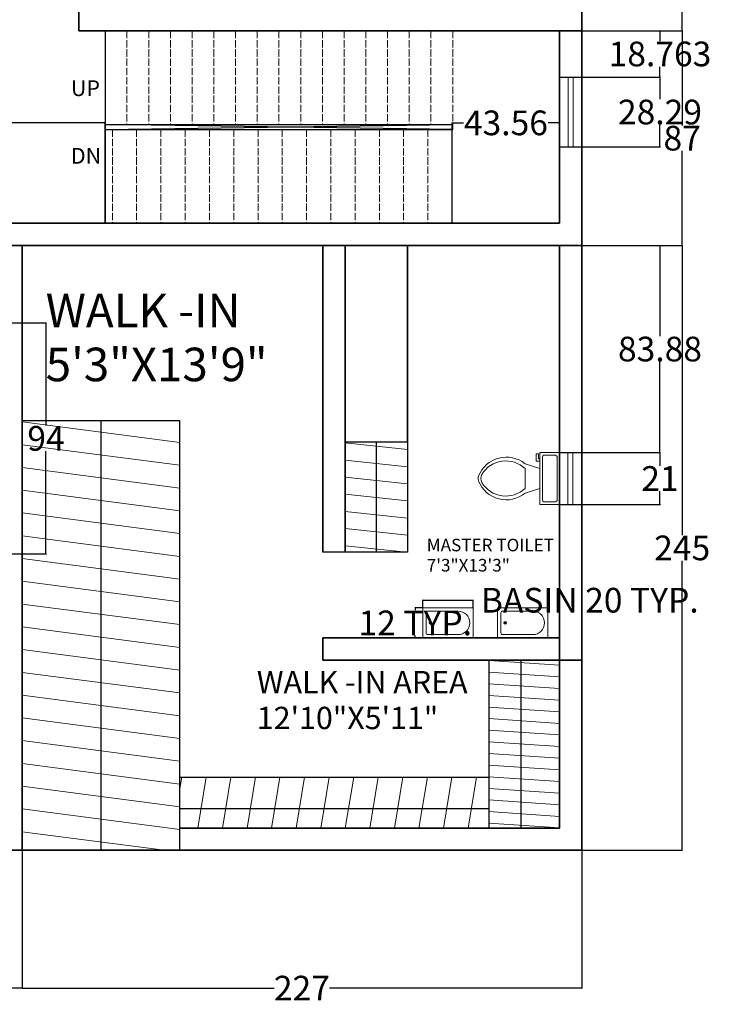
# Model space of a CAD drawing. Units: inches. Extents: x 135 to 880, y 60 to 879.
# Tile 3 of 5: x 557 to 838, y 60 to 459. Entities that reach past the tile are written whole.
import ezdxf

# ---------------------------------------------------------------- set-up
doc = ezdxf.new("R2010")
doc.units = ezdxf.units.IN
doc.header["$MEASUREMENT"] = 0
doc.linetypes.add('ACAD_ISO02W100', pattern=[15, 12, -3])
for name, color, linetype, lineweight in [('A-ANNO-DIMS', 2, 'Continuous', 18), ('A-ANNO-TEXT', 7, 'Continuous', 18), ('A-AREA-IDEN', 7, 'Continuous', 18), ('A-FLOR-CASE', 32, 'Continuous', 25), ('A-FLOR-CASE-PATT', 252, 'Continuous', 13), ('A-FLOR-FIXT', 9, 'Continuous', 20), ('A-FLOR-STRS', 7, 'Continuous', 25), ('A-FLOR-STRS-HIDN', 8, 'ACAD_ISO02W100', 18), ('A-GLAZ', 4, 'Continuous', 18), ('A-WALL', 7, 'Continuous', 35)]:
    doc.layers.add(name, color=color, linetype=linetype, lineweight=lineweight)
doc.styles.get("Standard").update_dxf_attribs({"font": 'arial.ttf'})
doc.dimstyles.get("Standard").update_dxf_attribs({"dimtxt": 10, "dimasz": 0.18, "dimexe": 0.18, "dimexo": 0.0625, "dimgap": 0.09, "dimtad": 0, "dimtih": 1, "dimtoh": 1, "dimdec": 0, "dimzin": 0, "dimdsep": 46, "dimlunit": 3, "dimtxsty": 'Standard', "dimcen": 0.09, "dimadec": 0, "dimazin": 0, "dimtfac": 1, "dimtdec": 0, "dimtofl": 0, "dimtmove": 0, "dimatfit": 3, "dimfxl": 1, "dimtolj": 1, "dimtzin": 0, "dimarcsym": 0})

# ---------------------------------------------------------------- blocks, each defined once
blk = doc.blocks.new('Toilet - top')
for p, q in [((9.5, -6), (9.5, -2)), ((-10, -8.5), (-8, -8.5)), ((-10, -9.5), (-10, -8.5)), ((-7, -9.5), (-10, -9.5)), ((-8, -8.5), (-8, -8)), ((-7, -8), (-7, -9.5)), ((-4, -8), (-6, -14)), ((4, -8), (6, -14)), ((4, -14), (-4, -14))]:
    blk.add_line(p, q)
blk.add_lwpolyline([(10.5, -8), (10.5, 0), (-10.5, 0), (-10.5, -8)], close=True)
for points in [[(-9.5, -2), (-9.5, -6)], [(8.5, -1), (-8.5, -1)], [(-8.5, -7), (8.5, -7)]]:
    blk.add_lwpolyline(points)
for centre, radius, start, end in [((-8.62, -1.88), 0.884, 81.8699, 188.1301), ((8.62, -1.88), 0.884, 351.8699, 98.1301), ((-8.62, -6.12), 0.884, 171.8699, 278.1301), ((8.62, -6.12), 0.884, 261.8699, 8.1301), ((3.52, -21.58), 12.17, 141.4691, 247.9714), ((4.2, -21.82), 11.33, 136.3677, 238.9468), ((-3.52, -21.58), 12.17, 292.0284, 38.5307), ((-4.2, -21.82), 11.33, 301.053, 43.6321), ((0, -27.88), 4, 245.7318, 294.2682), ((0, -29), 4, 254.8605, 285.1395)]:
    blk.add_arc(centre, radius, start, end)
blk = doc.blocks.new('Bath Tub - 26 x 60 in.')
for p, q in [((8, -18), (10, -18)), ((9, -17), (9, -19))]:
    blk.add_line(p, q)
blk.add_lwpolyline([(0, -36), (0, 0), (60, 0), (60, -36)], close=True)
for points in [[(4, -30), (4, -6)], [(6, -4), (42, -4)], [(42, -32), (6, -32)]]:
    blk.add_lwpolyline(points)
for radius in [1.5, 1]:
    blk.add_circle((9, -18), radius)
for centre, radius, start, end in [((5.75, -5.75), 1.77, 81.8699, 188.1301), ((42, -18), 14, 270, 90), ((5.75, -30.25), 1.77, 171.8699, 278.1301)]:
    blk.add_arc(centre, radius, start, end)
blk = doc.blocks.new('*D22')
at = {"layer": 'A-ANNO-DIMS', "color": 0, "lineweight": -2, "transparency": 16777216}
for p, q in [((720.5, 221.01), (720.5, 224.19)), ((720.68, 224.01), (740.73, 224.01)), ((740.91, 221.01), (740.91, 224.19)), ((740.91, 224.01), (741.09, 224.01))]:
    blk.add_line(p, q, dxfattribs=at)
at = {"layer": 'A-ANNO-DIMS', "color": 0, "transparency": 16777216}
for points in [[(720.68, 224.04), (720.68, 223.98), (720.5, 224.01)], [(740.73, 224.04), (740.73, 223.98), (740.91, 224.01)]]:
    blk.add_solid(points, dxfattribs=at)
at = {"layer": 'Defpoints', "color": 0, "transparency": 16777216}
for p in [(740.91, 224.01), (720.5, 220.95), (740.91, 220.95)]:
    blk.add_point(p, dxfattribs=at)
at = {"layer": 'A-ANNO-DIMS', "color": 0, "transparency": 16777216, "insert": (788.2, 224.01), "char_height": 10, "attachment_point": 5}
blk.add_mtext('\\A1;BASIN 20 TYP.', dxfattribs=at)
blk = doc.blocks.new('*D23')
at = {"layer": 'A-ANNO-DIMS', "color": 0, "lineweight": -2, "transparency": 16777216}
for p, q in [((720.44, 220.95), (717.26, 220.95)), ((717.44, 220.77), (717.44, 219.94)), ((720.44, 208.7), (717.26, 208.7)), ((717.44, 208.88), (717.44, 209.71))]:
    blk.add_line(p, q, dxfattribs=at)
at = {"layer": 'A-ANNO-DIMS', "color": 0, "transparency": 16777216}
for points in [[(717.41, 220.77), (717.47, 220.77), (717.44, 220.95)], [(717.41, 208.88), (717.47, 208.88), (717.44, 208.7)]]:
    blk.add_solid(points, dxfattribs=at)
at = {"layer": 'Defpoints', "color": 0, "transparency": 16777216}
for p in [(717.44, 220.95), (720.5, 220.95), (720.5, 208.7)]:
    blk.add_point(p, dxfattribs=at)
at = {"layer": 'A-ANNO-DIMS', "color": 0, "transparency": 16777216, "insert": (717.44, 214.82), "char_height": 10, "attachment_point": 5}
blk.add_mtext('\\A1;12 TYP.', dxfattribs=at)
blk = doc.blocks.new('*D27')
at = {"layer": 'A-ANNO-DIMS', "color": 0, "lineweight": -2, "transparency": 16777216}
for p, q in [((549.04, 336.39), (567.88, 336.39)), ((567.7, 336.21), (567.7, 294.78)), ((567.7, 242.96), (567.7, 284.39)), ((549.04, 242.78), (567.88, 242.78))]:
    blk.add_line(p, q, dxfattribs=at)
at = {"layer": 'A-ANNO-DIMS', "color": 0, "transparency": 16777216}
for points in [[(567.67, 336.21), (567.73, 336.21), (567.7, 336.39)], [(567.67, 242.96), (567.73, 242.96), (567.7, 242.78)]]:
    blk.add_solid(points, dxfattribs=at)
at = {"layer": 'Defpoints', "color": 0, "transparency": 16777216}
for p in [(548.98, 336.39), (548.98, 242.78), (567.7, 242.78)]:
    blk.add_point(p, dxfattribs=at)
at = {"layer": 'A-ANNO-DIMS', "color": 0, "transparency": 16777216, "insert": (567.7, 289.58), "char_height": 10, "attachment_point": 5}
blk.add_mtext('\\A1;94', dxfattribs=at)
blk = doc.blocks.new('*D55')
at = {"layer": 'A-ANNO-DIMS', "color": 0, "lineweight": -2, "transparency": 16777216}
for p, q in [((371.98, 122.64), (371.98, 66.67)), ((557.98, 122.64), (557.98, 66.67)), ((372.16, 66.85), (454.31, 66.85)), ((557.8, 66.85), (475.64, 66.85))]:
    blk.add_line(p, q, dxfattribs=at)
at = {"layer": 'A-ANNO-DIMS', "color": 0, "transparency": 16777216}
for points in [[(372.16, 66.88), (372.16, 66.82), (371.98, 66.85)], [(557.8, 66.88), (557.8, 66.82), (557.98, 66.85)]]:
    blk.add_solid(points, dxfattribs=at)
at = {"layer": 'Defpoints', "color": 0, "transparency": 16777216}
for p in [(371.98, 122.7), (557.98, 122.7), (557.98, 66.85)]:
    blk.add_point(p, dxfattribs=at)
at = {"layer": 'A-ANNO-DIMS', "color": 0, "transparency": 16777216, "insert": (464.98, 66.85), "char_height": 10, "attachment_point": 5}
blk.add_mtext('\\A1;186', dxfattribs=at)
blk = doc.blocks.new('*D56')
at = {"layer": 'A-ANNO-DIMS', "color": 0, "lineweight": -2, "transparency": 16777216}
for p, q in [((557.98, 122.64), (557.98, 66.67)), ((784.98, 122.64), (784.98, 66.67)), ((558.16, 66.85), (660.25, 66.85)), ((784.8, 66.85), (682.7, 66.85))]:
    blk.add_line(p, q, dxfattribs=at)
at = {"layer": 'A-ANNO-DIMS', "color": 0, "transparency": 16777216}
for points in [[(558.16, 66.88), (558.16, 66.82), (557.98, 66.85)], [(784.8, 66.88), (784.8, 66.82), (784.98, 66.85)]]:
    blk.add_solid(points, dxfattribs=at)
at = {"layer": 'Defpoints', "color": 0, "transparency": 16777216}
for p in [(557.98, 122.7), (784.98, 122.7), (784.98, 66.85)]:
    blk.add_point(p, dxfattribs=at)
at = {"layer": 'A-ANNO-DIMS', "color": 0, "transparency": 16777216, "insert": (671.48, 66.85), "char_height": 10, "attachment_point": 5}
blk.add_mtext('\\A1;227', dxfattribs=at)
blk = doc.blocks.new('*D61')
at = {"layer": 'A-ANNO-DIMS', "color": 0, "lineweight": -2, "transparency": 16777216}
for p, q in [((785.04, 367.7), (825.86, 367.7)), ((825.68, 367.52), (825.68, 250.4)), ((825.68, 122.88), (825.68, 240.01)), ((785.04, 122.7), (825.86, 122.7))]:
    blk.add_line(p, q, dxfattribs=at)
at = {"layer": 'A-ANNO-DIMS', "color": 0, "transparency": 16777216}
for points in [[(825.65, 367.52), (825.71, 367.52), (825.68, 367.7)], [(825.65, 122.88), (825.71, 122.88), (825.68, 122.7)]]:
    blk.add_solid(points, dxfattribs=at)
at = {"layer": 'Defpoints', "color": 0, "transparency": 16777216}
for p in [(784.98, 367.7), (825.68, 367.7), (784.98, 122.7)]:
    blk.add_point(p, dxfattribs=at)
at = {"layer": 'A-ANNO-DIMS', "color": 0, "transparency": 16777216, "insert": (825.68, 245.2), "char_height": 10, "attachment_point": 5}
blk.add_mtext('\\A1;245', dxfattribs=at)
blk = doc.blocks.new('*D62')
at = {"layer": 'A-ANNO-DIMS', "color": 0, "lineweight": -2, "transparency": 16777216}
for p, q in [((785.04, 454.7), (825.86, 454.7)), ((825.68, 454.52), (825.68, 416.4)), ((825.68, 367.88), (825.68, 406.01)), ((785.04, 367.7), (825.86, 367.7))]:
    blk.add_line(p, q, dxfattribs=at)
at = {"layer": 'A-ANNO-DIMS', "color": 0, "transparency": 16777216}
for points in [[(825.65, 454.52), (825.71, 454.52), (825.68, 454.7)], [(825.65, 367.88), (825.71, 367.88), (825.68, 367.7)]]:
    blk.add_solid(points, dxfattribs=at)
at = {"layer": 'Defpoints', "color": 0, "transparency": 16777216}
for p in [(784.98, 454.7), (825.68, 454.7), (784.98, 367.7)]:
    blk.add_point(p, dxfattribs=at)
at = {"layer": 'A-ANNO-DIMS', "color": 0, "transparency": 16777216, "insert": (825.68, 411.2), "char_height": 10, "attachment_point": 5}
blk.add_mtext('\\A1;87', dxfattribs=at)
blk = doc.blocks.new('*D63')
at = {"layer": 'A-ANNO-DIMS', "color": 0, "lineweight": -2, "transparency": 16777216}
for p, q in [((776.04, 545.7), (825.86, 545.7)), ((825.68, 545.52), (825.68, 505.4)), ((825.68, 454.88), (825.68, 495.01)), ((785.04, 454.7), (825.86, 454.7))]:
    blk.add_line(p, q, dxfattribs=at)
at = {"layer": 'A-ANNO-DIMS', "color": 0, "transparency": 16777216}
for points in [[(825.65, 545.52), (825.71, 545.52), (825.68, 545.7)], [(825.65, 454.88), (825.71, 454.88), (825.68, 454.7)]]:
    blk.add_solid(points, dxfattribs=at)
at = {"layer": 'Defpoints', "color": 0, "transparency": 16777216}
for p in [(775.98, 545.7), (825.68, 545.7), (784.98, 454.7)]:
    blk.add_point(p, dxfattribs=at)
at = {"layer": 'A-ANNO-DIMS', "color": 0, "transparency": 16777216, "insert": (825.68, 500.2), "char_height": 10, "attachment_point": 5}
blk.add_mtext('\\A1;91', dxfattribs=at)
blk = doc.blocks.new('*D66')
at = {"layer": 'A-ANNO-DIMS', "color": 0, "lineweight": -2, "transparency": 16777216}
for p, q in [((776.04, 367.7), (816.86, 367.7)), ((816.68, 367.52), (816.68, 330.96)), ((816.68, 284), (816.68, 320.56)), ((776.04, 283.82), (816.86, 283.82))]:
    blk.add_line(p, q, dxfattribs=at)
at = {"layer": 'A-ANNO-DIMS', "color": 0, "transparency": 16777216}
for points in [[(816.65, 367.52), (816.71, 367.52), (816.68, 367.7)], [(816.65, 284), (816.71, 284), (816.68, 283.82)]]:
    blk.add_solid(points, dxfattribs=at)
at = {"layer": 'Defpoints', "color": 0, "transparency": 16777216}
for p in [(775.98, 367.7), (775.98, 283.82), (816.68, 283.82)]:
    blk.add_point(p, dxfattribs=at)
at = {"layer": 'A-ANNO-DIMS', "color": 0, "transparency": 16777216, "insert": (816.68, 325.76), "char_height": 10, "attachment_point": 5}
blk.add_mtext('\\A1;83.88', dxfattribs=at)
blk = doc.blocks.new('*D67')
at = {"layer": 'A-ANNO-DIMS', "color": 0, "lineweight": -2, "transparency": 16777216}
for p, q in [((776.04, 283.82), (816.86, 283.82)), ((816.68, 283.64), (816.68, 278.43)), ((816.68, 263), (816.68, 268.21)), ((776.04, 262.82), (816.86, 262.82))]:
    blk.add_line(p, q, dxfattribs=at)
at = {"layer": 'A-ANNO-DIMS', "color": 0, "transparency": 16777216}
for points in [[(816.65, 283.64), (816.71, 283.64), (816.68, 283.82)], [(816.65, 263), (816.71, 263), (816.68, 262.82)]]:
    blk.add_solid(points, dxfattribs=at)
at = {"layer": 'Defpoints', "color": 0, "transparency": 16777216}
for p in [(775.98, 283.82), (775.98, 262.82), (816.68, 262.82)]:
    blk.add_point(p, dxfattribs=at)
at = {"layer": 'A-ANNO-DIMS', "color": 0, "transparency": 16777216, "insert": (816.68, 273.32), "char_height": 10, "attachment_point": 5}
blk.add_mtext('\\A1;21', dxfattribs=at)
blk = doc.blocks.new('*D68')
at = {"layer": 'A-ANNO-DIMS', "color": 0, "lineweight": -2, "transparency": 16777216}
for p, q in [((776.04, 454.7), (816.86, 454.7)), ((816.68, 454.52), (816.68, 450.52)), ((816.68, 436.12), (816.68, 440.12)), ((776.04, 435.94), (816.86, 435.94))]:
    blk.add_line(p, q, dxfattribs=at)
at = {"layer": 'A-ANNO-DIMS', "color": 0, "transparency": 16777216}
for points in [[(816.65, 454.52), (816.71, 454.52), (816.68, 454.7)], [(816.65, 436.12), (816.71, 436.12), (816.68, 435.94)]]:
    blk.add_solid(points, dxfattribs=at)
at = {"layer": 'Defpoints', "color": 0, "transparency": 16777216}
for p in [(775.98, 454.7), (775.98, 435.94), (816.68, 435.94)]:
    blk.add_point(p, dxfattribs=at)
at = {"layer": 'A-ANNO-DIMS', "color": 0, "transparency": 16777216, "insert": (816.68, 445.32), "char_height": 10, "attachment_point": 5}
blk.add_mtext('\\A1;18.763', dxfattribs=at)
blk = doc.blocks.new('*D69')
at = {"layer": 'A-ANNO-DIMS', "color": 0, "lineweight": -2, "transparency": 16777216}
for p, q in [((776.04, 435.94), (816.86, 435.94)), ((816.68, 435.76), (816.68, 426.99)), ((816.68, 407.83), (816.68, 416.6)), ((776.04, 407.65), (816.86, 407.65))]:
    blk.add_line(p, q, dxfattribs=at)
at = {"layer": 'A-ANNO-DIMS', "color": 0, "transparency": 16777216}
for points in [[(816.65, 435.76), (816.71, 435.76), (816.68, 435.94)], [(816.65, 407.83), (816.71, 407.83), (816.68, 407.65)]]:
    blk.add_solid(points, dxfattribs=at)
at = {"layer": 'Defpoints', "color": 0, "transparency": 16777216}
for p in [(775.98, 435.94), (775.98, 407.65), (816.68, 407.65)]:
    blk.add_point(p, dxfattribs=at)
at = {"layer": 'A-ANNO-DIMS', "color": 0, "transparency": 16777216, "insert": (816.68, 421.79), "char_height": 10, "attachment_point": 5}
blk.add_mtext('\\A1;28.29', dxfattribs=at)
blk = doc.blocks.new('*D74')
at = {"layer": 'A-ANNO-DIMS', "color": 0, "lineweight": -2, "transparency": 16777216}
for p, q in [((371.98, 376.76), (371.98, 417.58)), ((372.16, 417.4), (460.93, 417.4)), ((591.56, 417.4), (502.79, 417.4)), ((591.74, 376.76), (591.74, 417.58))]:
    blk.add_line(p, q, dxfattribs=at)
at = {"layer": 'A-ANNO-DIMS', "color": 0, "transparency": 16777216}
for points in [[(372.16, 417.43), (372.16, 417.37), (371.98, 417.4)], [(591.56, 417.43), (591.56, 417.37), (591.74, 417.4)]]:
    blk.add_solid(points, dxfattribs=at)
at = {"layer": 'Defpoints', "color": 0, "transparency": 16777216}
for p in [(591.74, 417.4), (371.98, 376.7), (591.74, 376.7)]:
    blk.add_point(p, dxfattribs=at)
at = {"layer": 'A-ANNO-DIMS', "color": 0, "transparency": 16777216, "insert": (481.86, 417.4), "char_height": 10, "attachment_point": 5}
blk.add_mtext('\\A1;219.76', dxfattribs=at)
blk = doc.blocks.new('*D75')
at = {"layer": 'A-ANNO-DIMS', "color": 0, "lineweight": -2, "transparency": 16777216}
for p, q in [((732.42, 376.76), (732.42, 417.58)), ((732.6, 417.4), (737.04, 417.4)), ((775.8, 417.4), (771.36, 417.4)), ((775.98, 376.76), (775.98, 417.58))]:
    blk.add_line(p, q, dxfattribs=at)
at = {"layer": 'A-ANNO-DIMS', "color": 0, "transparency": 16777216}
for points in [[(732.6, 417.43), (732.6, 417.37), (732.42, 417.4)], [(775.8, 417.43), (775.8, 417.37), (775.98, 417.4)]]:
    blk.add_solid(points, dxfattribs=at)
at = {"layer": 'Defpoints', "color": 0, "transparency": 16777216}
for p in [(775.98, 417.4), (732.42, 376.7), (775.98, 376.7)]:
    blk.add_point(p, dxfattribs=at)
at = {"layer": 'A-ANNO-DIMS', "color": 0, "transparency": 16777216, "insert": (754.2, 417.4), "char_height": 10, "attachment_point": 5}
blk.add_mtext('\\A1;43.56', dxfattribs=at)

msp = doc.modelspace()

# ---------------------------------------------------------------- hatches: boundary and pattern name
at = {"layer": 'A-FLOR-CASE-PATT'}
h = msp.add_hatch(dxfattribs=at)
h.set_pattern_fill('ANSI31', color=256, scale=73.16924, angle=127.5756, style=0)
h.paths.add_polyline_path([(583.7201, 122.7014), (621.9753, 122.7014), (621.9753, 292.0402), (586.2052, 296.7014), (557.9753, 296.7014), (557.9753, 126.0562)])
h = msp.add_hatch(dxfattribs=at)
h.set_pattern_fill('ANSI31', color=256, scale=55.2284, angle=128.93, style=0)
h.paths.add_polyline_path([(688.9753, 243.4405), (714.3091, 243.4405), (714.3091, 288.1752), (714.063, 288.2014), (688.9753, 288.2014)])
h = msp.add_hatch(dxfattribs=at)
h.set_pattern_fill('ANSI31', color=256, scale=37.5775, angle=131.1762, style=0)
h.paths.add_polyline_path([(747.2415, 131.7014), (775.9753, 131.7014), (775.9753, 199.7014), (747.2415, 199.7014)])
h = msp.add_hatch(dxfattribs=at)
h.set_pattern_fill('ANSI31', color=256, scale=78.639, angle=35.67, style=0)
h.paths.add_polyline_path([(621.9753, 131.7014), (743.3641, 131.7014), (746.7581, 152.3585), (621.9753, 152.3585)])

# ---------------------------------------------------------------- linework, layer by layer
at = {"layer": 'A-FLOR-CASE'}
for p, q in [((714.3091, 288.2014), (714.3091, 367.7014)), ((714.3091, 367.7014), (714.3091, 243.4405)), ((621.9753, 296.7014), (557.9753, 296.7014)), ((589.9753, 296.7014), (589.9753, 122.7014)), ((621.9753, 122.7014), (621.9753, 296.7014)), ((688.9753, 288.2014), (714.3091, 288.2014)), ((701.6422, 288.2014), (701.6422, 243.4405)), ((714.3091, 243.4405), (679.9753, 243.4405)), ((747.2415, 199.7014), (747.2415, 131.7014)), ((760.3963, 131.7014), (760.3963, 199.7014)), ((621.9753, 152.3585), (747.2415, 152.3585)), ((621.9753, 139.6868), (747.2415, 139.6868))]:
    msp.add_line(p, q, dxfattribs=at)
at = {"layer": 'A-FLOR-STRS'}
for p, q in [((591.7388, 454.7014), (591.7388, 376.7014)), ((591.7388, 416.7014), (732.6201, 416.7014)), ((732.6201, 414.7014), (591.7388, 416.7014)), ((591.7388, 414.7014), (732.6201, 416.7014)), ((732.6201, 414.7014), (732.6201, 416.7014)), ((591.7388, 414.7014), (732.6201, 414.7014))]:
    msp.add_line(p, q, dxfattribs=at)
at = {"layer": 'A-FLOR-STRS-HIDN', "ltscale": 0.25}
for p, q in [((591.7388, 454.7014), (591.7388, 416.7014)), ((600.5439, 454.7014), (600.5439, 416.7014)), ((609.349, 454.7014), (609.349, 416.7014)), ((618.154, 454.7014), (618.154, 416.7014)), ((626.9591, 454.7014), (626.9591, 416.7014)), ((635.7642, 454.7014), (635.7642, 416.7014)), ((644.5693, 454.7014), (644.5693, 416.7014)), ((653.3744, 454.7014), (653.3744, 416.7014)), ((662.1795, 454.7014), (662.1795, 416.7014)), ((670.9845, 454.7014), (670.9845, 416.7014)), ((679.7896, 454.7014), (679.7896, 416.7014)), ((688.5947, 454.7014), (688.5947, 416.7014)), ((697.3998, 454.7014), (697.3998, 416.7014)), ((706.2049, 454.7014), (706.2049, 416.7014)), ((715.01, 454.7014), (715.01, 416.7014)), ((723.815, 454.7014), (723.815, 416.7014)), ((732.6201, 454.7014), (732.6201, 416.7014)), ((594.6279, 414.7014), (594.6279, 376.7014)), ((604.47, 414.7014), (604.47, 376.7014)), ((614.312, 414.7014), (614.312, 376.7014)), ((624.1541, 414.7014), (624.1541, 376.7014)), ((633.9961, 414.7014), (633.9961, 376.7014)), ((643.8382, 414.7014), (643.8382, 376.7014)), ((653.6803, 414.7014), (653.6803, 376.7014)), ((663.5223, 414.7014), (663.5223, 376.7014)), ((673.3644, 414.7014), (673.3644, 376.7014)), ((683.2064, 414.7014), (683.2064, 376.7014)), ((693.0485, 414.7014), (693.0485, 376.7014)), ((702.8906, 414.7014), (702.8906, 376.7014)), ((712.7326, 414.7014), (712.7326, 376.7014)), ((722.5747, 414.7014), (722.5747, 376.7014)), ((732.4167, 414.7014), (732.4167, 376.7014))]:
    msp.add_line(p, q, dxfattribs=at)
at = {"layer": 'A-GLAZ'}
for p, q in [((775.9753, 435.9381), (784.9753, 435.9381)), ((779.4753, 435.9381), (779.4753, 407.6472)), ((781.4753, 435.9381), (781.4753, 407.6472)), ((775.9753, 407.6472), (784.9753, 407.6472)), ((775.9753, 283.8241), (784.7627, 283.8241)), ((779.369, 283.8241), (779.369, 262.8241)), ((781.369, 283.8241), (781.369, 262.8241)), ((775.9753, 262.8241), (784.9753, 262.8241))]:
    msp.add_line(p, q, dxfattribs=at)
at = {"layer": 'A-WALL'}
for p, q in [((580.9753, 454.7014), (580.9753, 536.7014)), ((784.9753, 536.7014), (784.9753, 454.7014)), ((784.9753, 454.7014), (580.9753, 454.7014)), ((784.9753, 454.7014), (669.9753, 454.7014)), ((775.9753, 376.7014), (775.9753, 454.7014)), ((784.9753, 367.7014), (784.9753, 454.7014)), ((775.9753, 376.7014), (371.9753, 376.7014)), ((784.9753, 367.7014), (371.9753, 367.7014)), ((548.9753, 367.7014), (557.9753, 367.7014)), ((557.9753, 122.7014), (557.9753, 367.7014)), ((679.9753, 243.4405), (679.9753, 367.7014)), ((688.9753, 243.4405), (688.9753, 367.7014)), ((775.9753, 367.7014), (775.9753, 208.7014)), ((784.9753, 367.7014), (784.9753, 199.7014)), ((775.9753, 208.7014), (679.9753, 208.7014)), ((679.9753, 199.7014), (679.9753, 208.7014)), ((775.9753, 208.7014), (775.9753, 199.7014)), ((784.9753, 199.7014), (679.9753, 199.7014)), ((775.9753, 199.7014), (775.9753, 131.7014)), ((784.9753, 199.7014), (784.9753, 122.7014)), ((775.9753, 131.7014), (621.9753, 131.7014)), ((371.9753, 122.7014), (557.9753, 122.7014)), ((784.9753, 122.7014), (557.9753, 122.7014))]:
    msp.add_line(p, q, dxfattribs=at)

# ---------------------------------------------------------------- block references
at = {"layer": 'A-FLOR-FIXT', "rotation": 270}
msp.add_blockref('Toilet - top', (775.9753, 273.3241), dxfattribs=at)
at = {"layer": 'A-FLOR-FIXT', "xscale": 0.3401549681485887, "yscale": 0.3401549681485887, "zscale": 0.3401549681485887}
for p in [(720.5018, 220.947), (750.8306, 220.947)]:
    msp.add_blockref('Bath Tub - 26 x 60 in.', p, dxfattribs=at)

# ---------------------------------------------------------------- texts
at = {"layer": 'A-ANNO-TEXT'}
for s, p in [('UP', (577.7849, 428.2549)), ('DN', (577.7849, 400.8582))]:
    msp.add_text(s, height=6.38926, dxfattribs=at).set_placement(p)
at = {"layer": 'A-AREA-IDEN'}
for s, height, p in [('WALK -IN ', 13.59119, (567.6001, 334.56)), ('5\'3"X13\'9"', 13.59119, (567.6001, 312.7269)), ('MASTER TOILET', 5.093493, (722.0918, 243.8168)), ('7\'3"X13\'3"', 5.09349, (722.0918, 235.6345)), ('WALK -IN AREA ', 9.045383, (653.1924, 186.3097)), ('12\'10"X5\'11"', 9.045383, (653.1924, 171.7791))]:
    msp.add_text(s, height=height, dxfattribs=at).set_placement(p)

# ---------------------------------------------------------------- dimensions: what is measured, and where the dimension line sits
at = {"layer": 'A-ANNO-DIMS'}
for base, p1, p2, angle, override, picture, middle in [((825.6753, 545.7014), (784.9753, 454.7014), (775.9753, 545.7014), 90, {"dimdec": 0, "dimlfac": 1, "dimrnd": 0, "dimzin": 0, "dimdsep": 46, "dimlunit": 2}, '*D63', (825.6753, 500.2014)), ((816.6753, 435.9381), (775.9753, 454.7014), (775.9753, 435.9381), 270, {"dimdec": 3, "dimlfac": 1, "dimrnd": 0, "dimzin": 0, "dimdsep": 46, "dimlunit": 2}, '*D68', (816.6753, 445.3198)), ((825.6753, 454.7014), (784.9753, 367.7014), (784.9753, 454.7014), 90, {"dimdec": 0, "dimlfac": 1, "dimrnd": 0, "dimzin": 0, "dimdsep": 46, "dimlunit": 2}, '*D62', (825.6753, 411.2014)), ((816.6753, 407.6472), (775.9753, 435.9381), (775.9753, 407.6472), 270, {"dimdec": 2, "dimlfac": 1, "dimrnd": 0, "dimzin": 0, "dimdsep": 46, "dimlunit": 2}, '*D69', (816.6753, 421.7927)), ((775.9753, 417.4014), (732.4167, 376.7014), (775.9753, 376.7014), 0, {"dimdec": 2, "dimlfac": 1, "dimrnd": 0, "dimzin": 0, "dimdsep": 46, "dimlunit": 2}, '*D75', (754.196, 417.4014)), ((816.6753, 283.8241), (775.9753, 367.7014), (775.9753, 283.8241), 270, {"dimdec": 2, "dimlfac": 1, "dimrnd": 0, "dimzin": 0, "dimdsep": 46, "dimlunit": 2}, '*D66', (816.6753, 325.7627)), ((825.6753, 367.7014), (784.9753, 122.7014), (784.9753, 367.7014), 90, {"dimdec": 0, "dimlfac": 1, "dimrnd": 0, "dimzin": 0, "dimdsep": 46, "dimlunit": 2}, '*D61', (825.6753, 245.2014)), ((567.6958, 242.7833), (548.9753, 336.3855), (548.9753, 242.7833), 270, {"dimdec": 0, "dimlfac": 1, "dimrnd": 0, "dimzin": 0, "dimdsep": 46, "dimlunit": 2}, '*D27', (567.6958, 289.5844)), ((816.6753, 262.8241), (775.9753, 283.8241), (775.9753, 262.8241), 270, {"dimdec": 0, "dimlfac": 1, "dimrnd": 0, "dimzin": 0, "dimdsep": 46, "dimlunit": 2}, '*D67', (816.6753, 273.3241))]:
    dim = msp.add_linear_dim(base=base, p1=p1, p2=p2, angle=angle, dimstyle='Standard', override=override, dxfattribs=at)
    dim.commit()
    dim.dimension.update_dxf_attribs({"geometry": picture, "text_midpoint": middle})
for base, p1, p2, override, picture, middle in [((591.7388, 417.4014), (371.9753, 376.7014), (591.7388, 376.7014), {"dimdec": 2, "dimlfac": 1, "dimrnd": 0, "dimzin": 0, "dimdsep": 46, "dimlunit": 2}, '*D74', (481.8571, 417.4014)), ((557.9753, 66.853), (371.9753, 122.7014), (557.9753, 122.7014), {"dimdec": 0, "dimlfac": 1, "dimrnd": 0, "dimzin": 0, "dimdsep": 46, "dimlunit": 2}, '*D55', (464.9753, 66.853)), ((784.9753, 66.853), (557.9753, 122.7014), (784.9753, 122.7014), {"dimdec": 0, "dimlfac": 1, "dimrnd": 0, "dimzin": 0, "dimdsep": 46, "dimlunit": 2}, '*D56', (671.4753, 66.853))]:
    dim = msp.add_linear_dim(base=base, p1=p1, p2=p2, dimstyle='Standard', override=override, dxfattribs=at)
    dim.commit()
    dim.dimension.update_dxf_attribs({"geometry": picture, "text_midpoint": middle})
dim = msp.add_linear_dim(base=(740.9111, 224.0084), p1=(720.5018, 220.947), p2=(740.9111, 220.947), text='BASIN <> TYP.', dimstyle='Standard', override={"dimdec": 0, "dimlfac": 1, "dimrnd": 0, "dimzin": 0, "dimdsep": 46, "dimlunit": 2}, dxfattribs=at)
dim.commit()
dim.dimension.update_dxf_attribs({"geometry": '*D22', "text_midpoint": (788.2002, 224.0084)})
dim = msp.add_linear_dim(base=(717.4404, 220.947), p1=(720.5018, 208.7014), p2=(720.5018, 220.947), angle=90, text='<> TYP.', dimstyle='Standard', override={"dimdec": 0, "dimlfac": 1, "dimrnd": 0, "dimzin": 0, "dimdsep": 46, "dimlunit": 2}, dxfattribs=at)
dim.commit()
dim.dimension.update_dxf_attribs({"geometry": '*D23', "text_midpoint": (717.4404, 214.8242)})

doc.saveas('drawing.dxf')
